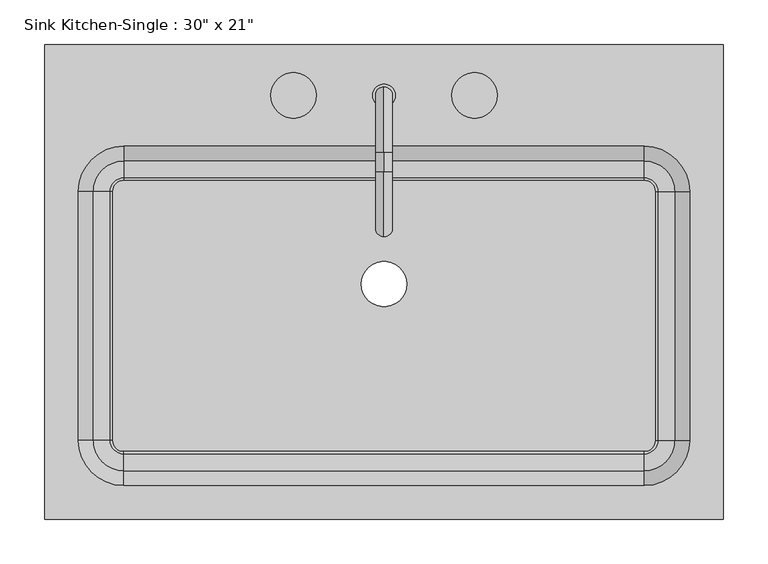
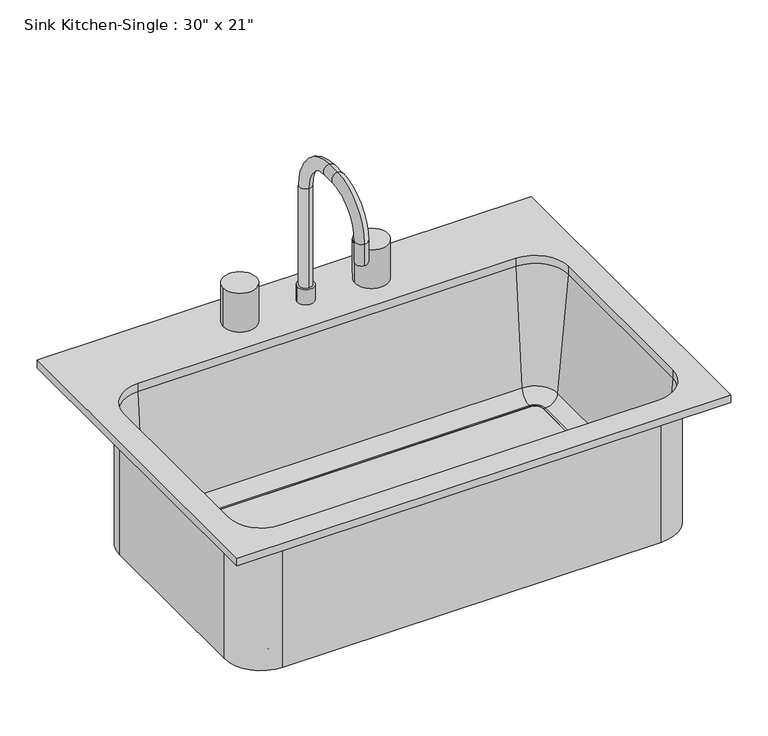
"""IFC4 building model written with IfcOpenShell, lengths in millimetres: flow terminal geometry."""

from ifc_helpers import new_model, si_unit, point, frame, frame_2d, origin, place, context, project, spatial, polyline, circle_curve, ellipse_curve, trimmed, segment, composite_curve, outline, extrude, source, transform, mapped, element, save
from ifc_brep_helpers import plane_surface, cylinder_surface, revolved_surface, advanced_brep


def flow_terminal_38af2918(model_context):
    return source(origin(), model_context, "Body", "SolidModel", [
        advanced_brep(
        [(396.6892406, 269.0454011, 927.1), (-365.3107594, 269.0454011, 927.1), (-365.3107594, -264.3545989, 927.1), (396.6892406, -264.3545989, 927.1), (307.7892406, 154.7454011, 927.1), (358.5892406, 103.9454011, 927.1), (358.5892406, -175.4545989, 927.1), (307.7892406, -226.2545989, 927.1), (-276.4107594, -226.2545989, 927.1), (-327.2107594, -175.4545989, 927.1), (-327.2107594, 103.9454011, 927.1), (-276.4107594, 154.7454011, 927.1), (396.6892406, 269.0454011, 914.4), (396.6892406, -264.3545989, 914.4), (-365.3107594, -264.3545989, 914.4), (-365.3107594, 269.0454011, 914.4), (364.9392406, 103.9454011, 914.4), (307.7892406, 161.0954011, 914.4), (-276.4107594, 161.0954011, 914.4), (-333.5607594, 103.9454011, 914.4), (-333.5607594, -175.4545989, 914.4), (-276.4107594, -232.6045989, 914.4), (307.7892406, -232.6045989, 914.4), (364.9392406, -175.4545989, 914.4), (307.7892406, 154.7454011, 914.4), (358.5892406, 103.9454011, 914.4), (358.5892406, -175.4545989, 914.4), (307.7892406, -226.2545989, 914.4), (-276.4107594, -226.2545989, 914.4), (-327.2107594, -175.4545989, 914.4), (-327.2107594, 103.9454011, 914.4), (-276.4107594, 154.7454011, 914.4), (364.9392406, 103.9454011, 698.5), (307.7892406, 161.0954011, 698.5), (320.4892406, 103.9454011, 698.5), (307.7892406, 116.6454011, 698.5), (320.4892406, 103.9454011, 708.025), (307.7892406, 116.6454011, 708.025), (323.0776588, 103.9454011, 708.025), (307.7892406, 119.2338193, 708.025), (342.0551678, 103.9454011, 725.4146831), (307.7892406, 138.2113283, 725.4146831), (364.9392406, -175.4545989, 698.5), (320.4892406, -175.4545989, 698.5), (320.4892406, -175.4545989, 708.025), (323.0776588, -175.4545989, 708.025), (342.0551678, -175.4545989, 725.4146831), (307.7892406, -232.6045989, 698.5), (307.7892406, -188.1545989, 698.5), (307.7892406, -188.1545989, 708.025), (307.7892406, -190.7430171, 708.025), (307.7892406, -209.7205261, 725.4146831), (-276.4107594, -232.6045989, 698.5), (-276.4107594, -188.1545989, 698.5), (-276.4107594, -188.1545989, 708.025), (-276.4107594, -190.7430171, 708.025), (-276.4107594, -209.7205261, 725.4146831), (-333.5607594, -175.4545989, 698.5), (-289.1107594, -175.4545989, 698.5), (-289.1107594, -175.4545989, 708.025), (-291.6991776, -175.4545989, 708.025), (-310.6766866, -175.4545989, 725.4146831), (-333.5607594, 103.9454011, 698.5), (-289.1107594, 103.9454011, 698.5), (-289.1107594, 103.9454011, 708.025), (-291.6991776, 103.9454011, 708.025), (-310.6766866, 103.9454011, 725.4146831), (-276.4107594, 161.0954011, 698.5), (-276.4107594, 116.6454011, 698.5), (-276.4107594, 116.6454011, 708.025), (-276.4107594, 119.2338193, 708.025), (-276.4107594, 138.2113283, 725.4146831)],
        [
            (0, 1),
            (1, 2),
            (2, 3),
            (3, 0),
            (4, 5, circle_curve(frame((307.7892406, 103.9454011, 927.1), z_axis=(0.0, 0.0, -1.0), x_axis=(1.0, 0.0, 0.0)), 50.8)),
            (5, 6),
            (6, 7, circle_curve(frame((307.7892406, -175.4545989, 927.1), z_axis=(0.0, 0.0, -1.0), x_axis=(1.0, 0.0, 0.0)), 50.8)),
            (7, 8),
            (8, 9, circle_curve(frame((-276.4107594, -175.4545989, 927.1), z_axis=(0.0, 0.0, -1.0), x_axis=(1.0, 0.0, 0.0)), 50.8)),
            (9, 10),
            (10, 11, circle_curve(frame((-276.4107594, 103.9454011, 927.1), z_axis=(0.0, 0.0, -1.0), x_axis=(1.0, 0.0, 0.0)), 50.8)),
            (11, 4),
            (12, 13),
            (13, 14),
            (14, 15),
            (15, 12),
            (16, 17, circle_curve(frame((307.7892406, 103.9454011, 914.4), z_axis=(0.0, 0.0, 1.0), x_axis=(0.0, 1.0, 0.0)), 57.15)),
            (17, 18),
            (18, 19, circle_curve(frame((-276.4107594, 103.9454011, 914.4), z_axis=(0.0, 0.0, 1.0), x_axis=(-1.0, 0.0, 0.0)), 57.15)),
            (19, 20),
            (20, 21, circle_curve(frame((-276.4107594, -175.4545989, 914.4), z_axis=(0.0, 0.0, 1.0), x_axis=(0.0, -1.0, 0.0)), 57.15)),
            (21, 22),
            (22, 23, circle_curve(frame((307.7892406, -175.4545989, 914.4), z_axis=(0.0, 0.0, 1.0), x_axis=(1.0, 0.0, 0.0)), 57.15)),
            (23, 16),
            (0, 12),
            (15, 1),
            (14, 2),
            (13, 3),
            (4, 24),
            (24, 25, circle_curve(frame((307.7892406, 103.9454011, 914.4), z_axis=(0.0, 0.0, -1.0), x_axis=(1.0, 0.0, 0.0)), 50.8)),
            (25, 5),
            (25, 26),
            (26, 6),
            (26, 27, circle_curve(frame((307.7892406, -175.4545989, 914.4), z_axis=(0.0, 0.0, -1.0), x_axis=(1.0, 0.0, 0.0)), 50.8)),
            (27, 7),
            (27, 28),
            (28, 8),
            (28, 29, circle_curve(frame((-276.4107594, -175.4545989, 914.4), z_axis=(0.0, 0.0, -1.0), x_axis=(1.0, 0.0, 0.0)), 50.8)),
            (29, 9),
            (29, 30),
            (30, 10),
            (30, 31, circle_curve(frame((-276.4107594, 103.9454011, 914.4), z_axis=(0.0, 0.0, -1.0), x_axis=(1.0, 0.0, 0.0)), 50.8)),
            (31, 11),
            (31, 24),
            (32, 33, circle_curve(frame((307.7892406, 103.9454011, 698.5), z_axis=(0.0, 0.0, 1.0), x_axis=(0.0, 1.0, 0.0)), 57.15)),
            (33, 17),
            (16, 32),
            (32, 34),
            (34, 35, circle_curve(frame((307.7892406, 103.9454011, 698.5), z_axis=(0.0, 0.0, 1.0), x_axis=(0.0, 1.0, 0.0)), 12.7)),
            (35, 33),
            (34, 36),
            (36, 37, circle_curve(frame((307.7892406, 103.9454011, 708.025), z_axis=(0.0, 0.0, 1.0), x_axis=(0.0, 1.0, 0.0)), 12.7)),
            (37, 35),
            (36, 38),
            (38, 39, circle_curve(frame((307.7892406, 103.9454011, 708.025), z_axis=(0.0, 0.0, 1.0), x_axis=(0.0, 1.0, 0.0)), 15.2884182)),
            (39, 37),
            (38, 40, circle_curve(frame((323.0776588, 103.9454011, 727.075), z_axis=(0.0, -1.0, 0.0), x_axis=(1.0, 0.0, 0.0)), 19.05)),
            (40, 41, circle_curve(frame((307.7892406, 103.9454011, 725.4146831), z_axis=(0.0, 0.0, 1.0), x_axis=(0.0, 1.0, 0.0)), 34.2659272)),
            (41, 39, circle_curve(frame((307.7892406, 119.2338193, 727.075), z_axis=(-1.0, 0.0, 0.0), x_axis=(0.0, 1.0, 0.0)), 19.05)),
            (40, 25),
            (24, 41),
            (23, 42),
            (42, 32),
            (42, 43),
            (43, 34),
            (43, 44),
            (44, 36),
            (44, 45),
            (45, 38),
            (45, 46, circle_curve(frame((323.0776588, -175.4545989, 727.075), z_axis=(0.0, -1.0, 0.0), x_axis=(1.0, 0.0, 0.0)), 19.05)),
            (46, 40),
            (46, 26),
            (22, 47),
            (47, 42, circle_curve(frame((307.7892406, -175.4545989, 698.5), z_axis=(0.0, 0.0, 1.0), x_axis=(1.0, 0.0, 0.0)), 57.15)),
            (47, 48),
            (48, 43, circle_curve(frame((307.7892406, -175.4545989, 698.5), z_axis=(0.0, 0.0, 1.0), x_axis=(1.0, 0.0, 0.0)), 12.7)),
            (48, 49),
            (49, 44, circle_curve(frame((307.7892406, -175.4545989, 708.025), z_axis=(0.0, 0.0, 1.0), x_axis=(1.0, 0.0, 0.0)), 12.7)),
            (49, 50),
            (50, 45, circle_curve(frame((307.7892406, -175.4545989, 708.025), z_axis=(0.0, 0.0, 1.0), x_axis=(1.0, 0.0, 0.0)), 15.2884182)),
            (50, 51, circle_curve(frame((307.7892406, -190.7430171, 727.075), z_axis=(-1.0, 0.0, 0.0), x_axis=(0.0, -1.0, 0.0)), 19.05)),
            (51, 46, circle_curve(frame((307.7892406, -175.4545989, 725.4146831), z_axis=(0.0, 0.0, 1.0), x_axis=(1.0, 0.0, 0.0)), 34.2659272)),
            (51, 27),
            (21, 52),
            (52, 47),
            (52, 53),
            (53, 48),
            (53, 54),
            (54, 49),
            (54, 55),
            (55, 50),
            (55, 56, circle_curve(frame((-276.4107594, -190.7430171, 727.075), z_axis=(-1.0, 0.0, 0.0), x_axis=(0.0, -1.0, 0.0)), 19.05)),
            (56, 51),
            (56, 28),
            (20, 57),
            (57, 52, circle_curve(frame((-276.4107594, -175.4545989, 698.5), z_axis=(0.0, 0.0, 1.0), x_axis=(0.0, -1.0, 0.0)), 57.15)),
            (57, 58),
            (58, 53, circle_curve(frame((-276.4107594, -175.4545989, 698.5), z_axis=(0.0, 0.0, 1.0), x_axis=(0.0, -1.0, 0.0)), 12.7)),
            (58, 59),
            (59, 54, circle_curve(frame((-276.4107594, -175.4545989, 708.025), z_axis=(0.0, 0.0, 1.0), x_axis=(0.0, -1.0, 0.0)), 12.7)),
            (59, 60),
            (60, 55, circle_curve(frame((-276.4107594, -175.4545989, 708.025), z_axis=(0.0, 0.0, 1.0), x_axis=(0.0, -1.0, 0.0)), 15.2884182)),
            (60, 61, circle_curve(frame((-291.6991776, -175.4545989, 727.075), z_axis=(0.0, 1.0, 0.0), x_axis=(-1.0, 0.0, 0.0)), 19.05)),
            (61, 56, circle_curve(frame((-276.4107594, -175.4545989, 725.4146831), z_axis=(0.0, 0.0, 1.0), x_axis=(0.0, -1.0, 0.0)), 34.2659272)),
            (61, 29),
            (19, 62),
            (62, 57),
            (62, 63),
            (63, 58),
            (63, 64),
            (64, 59),
            (64, 65),
            (65, 60),
            (65, 66, circle_curve(frame((-291.6991776, 103.9454011, 727.075), z_axis=(0.0, 1.0, 0.0), x_axis=(-1.0, 0.0, 0.0)), 19.05)),
            (66, 61),
            (66, 30),
            (18, 67),
            (67, 62, circle_curve(frame((-276.4107594, 103.9454011, 698.5), z_axis=(0.0, 0.0, 1.0), x_axis=(-1.0, 0.0, 0.0)), 57.15)),
            (67, 68),
            (68, 63, circle_curve(frame((-276.4107594, 103.9454011, 698.5), z_axis=(0.0, 0.0, 1.0), x_axis=(-1.0, 0.0, 0.0)), 12.7)),
            (68, 69),
            (69, 64, circle_curve(frame((-276.4107594, 103.9454011, 708.025), z_axis=(0.0, 0.0, 1.0), x_axis=(-1.0, 0.0, 0.0)), 12.7)),
            (69, 70),
            (70, 65, circle_curve(frame((-276.4107594, 103.9454011, 708.025), z_axis=(0.0, 0.0, 1.0), x_axis=(-1.0, 0.0, 0.0)), 15.2884182)),
            (70, 71, circle_curve(frame((-276.4107594, 119.2338193, 727.075), z_axis=(1.0, 0.0, 0.0), x_axis=(0.0, 1.0, 0.0)), 19.05)),
            (71, 66, circle_curve(frame((-276.4107594, 103.9454011, 725.4146831), z_axis=(0.0, 0.0, 1.0), x_axis=(-1.0, 0.0, 0.0)), 34.2659272)),
            (71, 31),
            (33, 67),
            (35, 68),
            (37, 69),
            (39, 70),
            (41, 71),
        ],
        [
            plane_surface(frame((-365.3107594, 269.0454011, 927.1), z_axis=(0.0, 0.0, 1.0), x_axis=(-1.0, 0.0, 0.0))),
            plane_surface(frame((-365.3107594, 269.0454011, 914.4), z_axis=(0.0, 0.0, -1.0), x_axis=(1.0, 0.0, 0.0))),
            plane_surface(frame((396.6892406, 269.0454011, 927.1), z_axis=(0.0, 1.0, 0.0), x_axis=(0.0, 0.0, -1.0))),
            plane_surface(frame((-365.3107594, 269.0454011, 927.1), z_axis=(-1.0, 0.0, 0.0), x_axis=(0.0, 0.0, -1.0))),
            plane_surface(frame((-365.3107594, -264.3545989, 927.1), z_axis=(0.0, -1.0, 0.0), x_axis=(0.0, 0.0, -1.0))),
            plane_surface(frame((396.6892406, -264.3545989, 927.1), z_axis=(1.0, 0.0, 0.0), x_axis=(0.0, 0.0, -1.0))),
            revolved_surface(polyline([(358.58924060000004, 103.9454011, 914.4), (358.58924060000004, 103.9454011, 927.1)]), (307.7892406, 103.9454011, 0.0), (0.0, 0.0, -1.0)),
            plane_surface(frame((358.5892406, 103.9454011, 927.1), z_axis=(-1.0, 0.0, 0.0), x_axis=(0.0, 0.0, -1.0))),
            revolved_surface(polyline([(358.58924060000004, -175.4545989, 914.4), (358.58924060000004, -175.4545989, 927.1)]), (307.7892406, -175.4545989, 0.0), (0.0, 0.0, -1.0)),
            plane_surface(frame((307.7892406, -226.2545989, 927.1), z_axis=(0.0, 1.0, 0.0), x_axis=(0.0, 0.0, -1.0))),
            revolved_surface(polyline([(-225.6107594, -175.4545989, 914.4), (-225.6107594, -175.4545989, 927.1)]), (-276.4107594, -175.4545989, 0.0), (0.0, 0.0, -1.0)),
            plane_surface(frame((-327.2107594, -175.4545989, 927.1), z_axis=(1.0, 0.0, 0.0), x_axis=(0.0, 0.0, -1.0))),
            revolved_surface(polyline([(-225.6107594, 103.9454011, 914.4), (-225.6107594, 103.9454011, 927.1)]), (-276.4107594, 103.9454011, 0.0), (0.0, 0.0, -1.0)),
            plane_surface(frame((-276.4107594, 154.7454011, 927.1), z_axis=(0.0, -1.0, 0.0), x_axis=(0.0, 0.0, -1.0))),
            cylinder_surface(frame((307.7892406, 103.9454011, 0.0), z_axis=(0.0, 0.0, -1.0), x_axis=(0.0, 1.0, 0.0)), 57.15),
            plane_surface(frame((307.7892406, 103.9454011, 698.5), z_axis=(0.0, 0.0, -1.0), x_axis=(0.0, 1.0, 0.0))),
            revolved_surface(polyline([(307.7892406, 116.6454011, 698.5), (307.7892406, 116.6454011, 708.025)]), (307.7892406, 103.9454011, 0.0), (0.0, 0.0, -1.0)),
            plane_surface(frame((307.7892406, 103.9454011, 708.025), z_axis=(0.0, 0.0, 1.0), x_axis=(0.0, 1.0, 0.0))),
            revolved_surface(trimmed(ellipse_curve(frame((307.7892406, 119.2338193, 727.075), z_axis=(1.0, 0.0, 0.0), x_axis=(0.0, 1.0, 0.0)), 19.05, 19.05), [point((307.7892406, 119.2338193, 708.025))], [point((307.7892406, 138.2113283, 725.4146831))], True, "CARTESIAN"), (307.7892406, 103.9454011, 0.0), (0.0, 0.0, -1.0)),
            revolved_surface(polyline([(307.7892406, 138.2113283, 725.4146831), (307.7892406, 154.7454011, 914.4)]), (307.7892406, 103.9454011, 0.0), (0.0, 0.0, -1.0)),
            plane_surface(frame((364.9392406, 103.9454011, 914.4), z_axis=(1.0, 0.0, 0.0), x_axis=(0.0, -1.0, 0.0))),
            plane_surface(frame((364.9392406, 103.9454011, 698.5), z_axis=(0.0, 0.0, -1.0), x_axis=(0.0, -1.0, 0.0))),
            plane_surface(frame((320.4892406, 103.9454011, 698.5), z_axis=(-1.0, 0.0, 0.0), x_axis=(0.0, -1.0, 0.0))),
            plane_surface(frame((320.4892406, 103.9454011, 708.025), z_axis=(0.0, 0.0, 1.0), x_axis=(0.0, -1.0, 0.0))),
            revolved_surface(polyline([(342.1276588, -175.45459889999998, 727.075), (342.1276588, 103.9454011, 727.075)]), (323.0776588, 103.9454011, 727.075), (0.0, -1.0, 0.0)),
            plane_surface(frame((342.0551678, 103.9454011, 725.4146831), z_axis=(-0.9961946980917442, 0.0, 0.08715574274767306), x_axis=(0.0, -1.0, 0.0))),
            cylinder_surface(frame((307.7892406, -175.4545989, 0.0), z_axis=(0.0, 0.0, -1.0), x_axis=(1.0, 0.0, 0.0)), 57.15),
            plane_surface(frame((307.7892406, -175.4545989, 698.5), z_axis=(0.0, 0.0, -1.0), x_axis=(1.0, 0.0, 0.0))),
            revolved_surface(polyline([(320.4892406, -175.4545989, 698.5), (320.4892406, -175.4545989, 708.025)]), (307.7892406, -175.4545989, 0.0), (0.0, 0.0, -1.0)),
            plane_surface(frame((307.7892406, -175.4545989, 708.025), z_axis=(0.0, 0.0, 1.0), x_axis=(1.0, 0.0, 0.0))),
            revolved_surface(trimmed(ellipse_curve(frame((323.0776588, -175.4545989, 727.075), z_axis=(0.0, -1.0, 0.0), x_axis=(1.0, 0.0, 0.0)), 19.05, 19.05), [point((323.0776588, -175.4545989, 708.025))], [point((342.0551678, -175.4545989, 725.4146831))], True, "CARTESIAN"), (307.7892406, -175.4545989, 0.0), (0.0, 0.0, -1.0)),
            revolved_surface(polyline([(342.0551678, -175.4545989, 725.4146831), (358.5892406, -175.4545989, 914.4)]), (307.7892406, -175.4545989, 0.0), (0.0, 0.0, -1.0)),
            plane_surface(frame((307.7892406, -232.6045989, 914.4), z_axis=(0.0, -1.0, 0.0), x_axis=(-1.0, 0.0, 0.0))),
            plane_surface(frame((307.7892406, -232.6045989, 698.5), z_axis=(0.0, 0.0, -1.0), x_axis=(-1.0, 0.0, 0.0))),
            plane_surface(frame((307.7892406, -188.1545989, 698.5), z_axis=(0.0, 1.0, 0.0), x_axis=(-1.0, 0.0, 0.0))),
            plane_surface(frame((307.7892406, -188.1545989, 708.025), z_axis=(0.0, 0.0, 1.0), x_axis=(-1.0, 0.0, 0.0))),
            revolved_surface(polyline([(-276.4107594, -209.79301710000001, 727.075), (307.7892406, -209.79301710000001, 727.075)]), (307.7892406, -190.7430171, 727.075), (-1.0, 0.0, 0.0)),
            plane_surface(frame((307.7892406, -209.7205261, 725.4146831), z_axis=(0.0, 0.9961946980917442, 0.08715574274767306), x_axis=(-1.0, 0.0, 0.0))),
            cylinder_surface(frame((-276.4107594, -175.4545989, 0.0), z_axis=(0.0, 0.0, -1.0), x_axis=(0.0, -1.0, 0.0)), 57.15),
            plane_surface(frame((-276.4107594, -175.4545989, 698.5), z_axis=(0.0, 0.0, -1.0), x_axis=(0.0, -1.0, 0.0))),
            revolved_surface(polyline([(-276.4107594, -188.1545989, 698.5), (-276.4107594, -188.1545989, 708.025)]), (-276.4107594, -175.4545989, 0.0), (0.0, 0.0, -1.0)),
            plane_surface(frame((-276.4107594, -175.4545989, 708.025), z_axis=(0.0, 0.0, 1.0), x_axis=(0.0, -1.0, 0.0))),
            revolved_surface(trimmed(ellipse_curve(frame((-276.4107594, -190.7430171, 727.075), z_axis=(-1.0, 0.0, 0.0), x_axis=(0.0, -1.0, 0.0)), 19.05, 19.05), [point((-276.4107594, -190.7430171, 708.025))], [point((-276.4107594, -209.7205261, 725.4146831))], True, "CARTESIAN"), (-276.4107594, -175.4545989, 0.0), (0.0, 0.0, -1.0)),
            revolved_surface(polyline([(-276.4107594, -209.7205261, 725.4146831), (-276.4107594, -226.2545989, 914.4)]), (-276.4107594, -175.4545989, 0.0), (0.0, 0.0, -1.0)),
            plane_surface(frame((-333.5607594, -175.4545989, 914.4), z_axis=(-1.0, 0.0, 0.0), x_axis=(0.0, 1.0, 0.0))),
            plane_surface(frame((-333.5607594, -175.4545989, 698.5), z_axis=(0.0, 0.0, -1.0), x_axis=(0.0, 1.0, 0.0))),
            plane_surface(frame((-289.1107594, -175.4545989, 698.5), z_axis=(1.0, 0.0, 0.0), x_axis=(0.0, 1.0, 0.0))),
            plane_surface(frame((-289.1107594, -175.4545989, 708.025), z_axis=(0.0, 0.0, 1.0), x_axis=(0.0, 1.0, 0.0))),
            revolved_surface(polyline([(-310.7491776, 103.94540109999997, 727.075), (-310.7491776, -175.4545989, 727.075)]), (-291.6991776, -175.4545989, 727.075), (0.0, 1.0, 0.0)),
            plane_surface(frame((-310.6766866, -175.4545989, 725.4146831), z_axis=(0.9961946980917442, 0.0, 0.08715574274767306), x_axis=(0.0, 1.0, 0.0))),
            cylinder_surface(frame((-276.4107594, 103.9454011, 0.0), z_axis=(0.0, 0.0, -1.0), x_axis=(-1.0, 0.0, 0.0)), 57.15),
            plane_surface(frame((-276.4107594, 103.9454011, 698.5), z_axis=(0.0, 0.0, -1.0), x_axis=(-1.0, 0.0, 0.0))),
            revolved_surface(polyline([(-289.1107594, 103.9454011, 698.5), (-289.1107594, 103.9454011, 708.025)]), (-276.4107594, 103.9454011, 0.0), (0.0, 0.0, -1.0)),
            plane_surface(frame((-276.4107594, 103.9454011, 708.025), z_axis=(0.0, 0.0, 1.0), x_axis=(-1.0, 0.0, 0.0))),
            revolved_surface(trimmed(ellipse_curve(frame((-291.6991776, 103.9454011, 727.075), z_axis=(0.0, 1.0, 0.0), x_axis=(-1.0, 0.0, 0.0)), 19.05, 19.05), [point((-291.6991776, 103.9454011, 708.025))], [point((-310.6766866, 103.9454011, 725.4146831))], True, "CARTESIAN"), (-276.4107594, 103.9454011, 0.0), (0.0, 0.0, -1.0)),
            revolved_surface(polyline([(-310.6766866, 103.9454011, 725.4146831), (-327.2107594, 103.9454011, 914.4)]), (-276.4107594, 103.9454011, 0.0), (0.0, 0.0, -1.0)),
            plane_surface(frame((-276.4107594, 161.0954011, 914.4), z_axis=(0.0, 1.0, 0.0), x_axis=(1.0, 0.0, 0.0))),
            plane_surface(frame((-276.4107594, 161.0954011, 698.5), z_axis=(0.0, 0.0, -1.0), x_axis=(1.0, 0.0, 0.0))),
            plane_surface(frame((-276.4107594, 116.6454011, 698.5), z_axis=(0.0, -1.0, 0.0), x_axis=(1.0, 0.0, 0.0))),
            plane_surface(frame((-276.4107594, 116.6454011, 708.025), z_axis=(0.0, 0.0, 1.0), x_axis=(1.0, 0.0, 0.0))),
            revolved_surface(polyline([(307.7892406, 138.2838193, 727.075), (-276.4107594, 138.2838193, 727.075)]), (-276.4107594, 119.2338193, 727.075), (1.0, 0.0, 0.0)),
            plane_surface(frame((-276.4107594, 138.2113283, 725.4146831), z_axis=(0.0, -0.9961946980917442, 0.08715574274767306), x_axis=(1.0, 0.0, 0.0))),
        ],
        [
            (0, [[1, 2, 3, 4], [5, 6, 7, 8, 9, 10, 11, 12]]),
            (1, [[13, 14, 15, 16], [17, 18, 19, 20, 21, 22, 23, 24]]),
            (2, [[-1, 25, -16, 26]]),
            (3, [[-2, -26, -15, 27]]),
            (4, [[-3, -27, -14, 28]]),
            (5, [[-4, -28, -13, -25]]),
            (6, [[-5, 29, 30, 31]]),
            (7, [[-6, -31, 32, 33]]),
            (8, [[-7, -33, 34, 35]]),
            (9, [[-8, -35, 36, 37]]),
            (10, [[-9, -37, 38, 39]]),
            (11, [[-10, -39, 40, 41]]),
            (12, [[-11, -41, 42, 43]]),
            (13, [[-12, -43, 44, -29]]),
            (14, [[45, 46, -17, 47]]),
            (15, [[-45, 48, 49, 50]]),
            (16, [[-49, 51, 52, 53]]),
            (17, [[-52, 54, 55, 56]]),
            (18, [[-55, 57, 58, 59]]),
            (19, [[-58, 60, -30, 61]]),
            (20, [[-47, -24, 62, 63]]),
            (21, [[-48, -63, 64, 65]]),
            (22, [[-51, -65, 66, 67]]),
            (23, [[-54, -67, 68, 69]]),
            (24, [[-57, -69, 70, 71]]),
            (25, [[-60, -71, 72, -32]]),
            (26, [[-62, -23, 73, 74]]),
            (27, [[-64, -74, 75, 76]]),
            (28, [[-66, -76, 77, 78]]),
            (29, [[-68, -78, 79, 80]]),
            (30, [[-70, -80, 81, 82]]),
            (31, [[-72, -82, 83, -34]]),
            (32, [[-73, -22, 84, 85]]),
            (33, [[-75, -85, 86, 87]]),
            (34, [[-77, -87, 88, 89]]),
            (35, [[-79, -89, 90, 91]]),
            (36, [[-81, -91, 92, 93]]),
            (37, [[-83, -93, 94, -36]]),
            (38, [[-84, -21, 95, 96]]),
            (39, [[-86, -96, 97, 98]]),
            (40, [[-88, -98, 99, 100]]),
            (41, [[-90, -100, 101, 102]]),
            (42, [[-92, -102, 103, 104]]),
            (43, [[-94, -104, 105, -38]]),
            (44, [[-95, -20, 106, 107]]),
            (45, [[-97, -107, 108, 109]]),
            (46, [[-99, -109, 110, 111]]),
            (47, [[-101, -111, 112, 113]]),
            (48, [[-103, -113, 114, 115]]),
            (49, [[-105, -115, 116, -40]]),
            (50, [[-106, -19, 117, 118]]),
            (51, [[-108, -118, 119, 120]]),
            (52, [[-110, -120, 121, 122]]),
            (53, [[-112, -122, 123, 124]]),
            (54, [[-114, -124, 125, 126]]),
            (55, [[-116, -126, 127, -42]]),
            (56, [[-46, 128, -117, -18]]),
            (57, [[-50, 129, -119, -128]]),
            (58, [[-53, 130, -121, -129]]),
            (59, [[-56, 131, -123, -130]]),
            (60, [[-59, 132, -125, -131]]),
            (61, [[-61, -44, -127, -132]]),
        ],
    ),
        advanced_brep(
        [(2.9892406, 211.8954011, 927.1), (28.3892406, 211.8954011, 927.1), (15.6892406, 221.4204011, 1114.425), (15.6892406, 202.3704011, 1114.425), (15.6892406, 202.3704011, 952.5), (15.6892406, 221.4204011, 952.5), (15.6892406, 148.3954011, 1187.45), (15.6892406, 148.3954011, 1168.4), (15.6892406, 126.1704011, 1187.45), (15.6892406, 126.1704011, 1168.4), (15.6892406, 53.1454011, 1114.425), (15.6892406, 72.1954011, 1114.425), (15.6892406, 53.1454011, 1079.5), (15.6892406, 72.1954011, 1079.5), (2.9892406, 211.8954011, 952.5), (28.3892406, 211.8954011, 952.5)],
        [
            (0, 1, circle_curve(frame((15.6892406, 211.8954011, 927.1), z_axis=(0.0, 0.0, -1.0), x_axis=(1.0, 0.0, 0.0)), 12.7)),
            (1, 0, circle_curve(frame((15.6892406, 211.8954011, 927.1), z_axis=(0.0, 0.0, -1.0), x_axis=(1.0, 0.0, 0.0)), 12.7)),
            (2, 3, circle_curve(frame((15.6892406, 211.8954011, 1114.425), z_axis=(0.0, 0.0, -1.0), x_axis=(0.0, -1.0, 0.0)), 9.525)),
            (3, 4),
            (4, 5, circle_curve(frame((15.6892406, 211.8954011, 952.5), z_axis=(0.0, 0.0, 1.0), x_axis=(0.0, -1.0, 0.0)), 9.525)),
            (5, 2),
            (3, 2, circle_curve(frame((15.6892406, 211.8954011, 1114.425), z_axis=(0.0, 0.0, -1.0), x_axis=(0.0, -1.0, 0.0)), 9.525)),
            (5, 4, circle_curve(frame((15.6892406, 211.8954011, 952.5), z_axis=(0.0, 0.0, 1.0), x_axis=(0.0, -1.0, 0.0)), 9.525)),
            (2, 6, circle_curve(frame((15.6892406, 148.3954011, 1114.425), z_axis=(1.0, 0.0, 0.0), x_axis=(0.0, 1.0, 0.0)), 73.025)),
            (6, 7, circle_curve(frame((15.6892406, 148.3954011, 1177.925), z_axis=(0.0, 1.0, 0.0), x_axis=(0.0, 0.0, -1.0)), 9.525)),
            (7, 3, circle_curve(frame((15.6892406, 148.3954011, 1114.425), z_axis=(-1.0, 0.0, 0.0), x_axis=(0.0, 1.0, 0.0)), 53.975)),
            (7, 6, circle_curve(frame((15.6892406, 148.3954011, 1177.925), z_axis=(0.0, 1.0, 0.0), x_axis=(0.0, 0.0, -1.0)), 9.525)),
            (6, 8),
            (8, 9, circle_curve(frame((15.6892406, 126.1704011, 1177.925), z_axis=(0.0, 1.0, 0.0), x_axis=(0.0, 0.0, -1.0)), 9.525)),
            (9, 7),
            (9, 8, circle_curve(frame((15.6892406, 126.1704011, 1177.925), z_axis=(0.0, 1.0, 0.0), x_axis=(0.0, 0.0, -1.0)), 9.525)),
            (8, 10, circle_curve(frame((15.6892406, 126.1704011, 1114.425), z_axis=(1.0, 0.0, 0.0), x_axis=(0.0, 0.0, 1.0)), 73.025)),
            (10, 11, circle_curve(frame((15.6892406, 62.6704011, 1114.425), z_axis=(0.0, 0.0, 1.0), x_axis=(0.0, 1.0, 0.0)), 9.525)),
            (11, 9, circle_curve(frame((15.6892406, 126.1704011, 1114.425), z_axis=(-1.0, 0.0, 0.0), x_axis=(0.0, 0.0, 1.0)), 53.975)),
            (11, 10, circle_curve(frame((15.6892406, 62.6704011, 1114.425), z_axis=(0.0, 0.0, 1.0), x_axis=(0.0, 1.0, 0.0)), 9.525)),
            (12, 13, circle_curve(frame((15.6892406, 62.6704011, 1079.5), z_axis=(0.0, 0.0, -1.0), x_axis=(0.0, 1.0, 0.0)), 9.525)),
            (13, 12, circle_curve(frame((15.6892406, 62.6704011, 1079.5), z_axis=(0.0, 0.0, -1.0), x_axis=(0.0, 1.0, 0.0)), 9.525)),
            (10, 12),
            (13, 11),
            (14, 15, circle_curve(frame((15.6892406, 211.8954011, 952.5), z_axis=(0.0, 0.0, 1.0), x_axis=(1.0, 0.0, 0.0)), 12.7)),
            (15, 14, circle_curve(frame((15.6892406, 211.8954011, 952.5), z_axis=(0.0, 0.0, 1.0), x_axis=(1.0, 0.0, 0.0)), 12.7)),
            (14, 0),
            (1, 15),
        ],
        [
            plane_surface(frame((15.6892406, 202.3704011, 927.1), z_axis=(0.0, 0.0, -1.0), x_axis=(1.0, 0.0, 0.0))),
            cylinder_surface(frame((15.6892406, 211.8954011, 927.1), z_axis=(0.0, 0.0, -1.0), x_axis=(0.0, -1.0, 0.0)), 9.525),
            revolved_surface(trimmed(ellipse_curve(frame((15.6892406, 211.8954011, 1114.425), z_axis=(0.0, 0.0, -1.0), x_axis=(0.0, -1.0, 0.0)), 9.525, 9.525), [point((15.6892406, 221.4204011, 1114.425))], [point((15.6892406, 202.3704011, 1114.425))], True, "CARTESIAN"), (15.6892406, 148.3954011, 1114.425), (1.0, 0.0, 0.0)),
            revolved_surface(trimmed(ellipse_curve(frame((15.6892406, 211.8954011, 1114.425), z_axis=(0.0, 0.0, -1.0), x_axis=(0.0, -1.0, 0.0)), 9.525, 9.525), [point((15.6892406, 202.3704011, 1114.425))], [point((15.6892406, 221.4204011, 1114.425))], True, "CARTESIAN"), (15.6892406, 148.3954011, 1114.425), (1.0, 0.0, 0.0)),
            cylinder_surface(frame((15.6892406, 148.3954011, 1177.925), z_axis=(0.0, 1.0, 0.0), x_axis=(0.0, 0.0, -1.0)), 9.525),
            revolved_surface(trimmed(ellipse_curve(frame((15.6892406, 126.1704011, 1177.925), z_axis=(0.0, 1.0, 0.0), x_axis=(0.0, 0.0, -1.0)), 9.525, 9.525), [point((15.6892406, 126.1704011, 1187.45))], [point((15.6892406, 126.1704011, 1168.4))], True, "CARTESIAN"), (15.6892406, 126.1704011, 1114.425), (1.0, 0.0, 0.0)),
            revolved_surface(trimmed(ellipse_curve(frame((15.6892406, 126.1704011, 1177.925), z_axis=(0.0, 1.0, 0.0), x_axis=(0.0, 0.0, -1.0)), 9.525, 9.525), [point((15.6892406, 126.1704011, 1168.4))], [point((15.6892406, 126.1704011, 1187.45))], True, "CARTESIAN"), (15.6892406, 126.1704011, 1114.425), (1.0, 0.0, 0.0)),
            plane_surface(frame((15.6892406, 53.1454011, 1079.5), z_axis=(0.0, 0.0, -1.0), x_axis=(-1.0, 0.0, 0.0))),
            cylinder_surface(frame((15.6892406, 62.6704011, 1114.425), z_axis=(0.0, 0.0, 1.0), x_axis=(0.0, 1.0, 0.0)), 9.525),
            plane_surface(frame((28.3892406, 211.8954011, 952.5), z_axis=(0.0, 0.0, 1.0), x_axis=(0.0, 1.0, 0.0))),
            cylinder_surface(frame((15.6892406, 211.8954011, 927.1), z_axis=(0.0, 0.0, 1.0), x_axis=(1.0, 0.0, 0.0)), 12.7),
        ],
        [
            (0, [[1, 2]]),
            (1, [[3, 4, 5, 6]]),
            (1, [[7, -6, 8, -4]]),
            (2, [[-3, 9, 10, 11]]),
            (3, [[-7, -11, 12, -9]]),
            (4, [[-10, 13, 14, 15]]),
            (4, [[-12, -15, 16, -13]]),
            (5, [[-14, 17, 18, 19]]),
            (6, [[-16, -19, 20, -17]]),
            (7, [[21, 22]]),
            (8, [[-18, 23, -22, 24]]),
            (8, [[-20, -24, -21, -23]]),
            (9, [[25, 26], [-5, -8]]),
            (10, [[-25, 27, -2, 28]]),
            (10, [[-26, -28, -1, -27]]),
        ],
    ),
        extrude(outline(composite_curve([segment(trimmed(circle_curve(frame_2d((-85.9107594, 211.8954011)), 25.4), [point((-111.3107594, 211.8954011))], [point((-60.5107594, 211.8954011))], False, "CARTESIAN"), True, "CONTINUOUS"), segment(trimmed(circle_curve(frame_2d((-85.9107594, 211.8954011)), 25.4), [point((-60.5107594, 211.8954011))], [point((-111.3107594, 211.8954011))], False, "CARTESIAN"), True, "CONTINUOUS")], self_intersect=False)), frame((0.0, 0.0, 927.1), z_axis=(0.0, 0.0, 1.0), x_axis=(1.0, 0.0, 0.0)), (0.0, 0.0, 1.0), 63.5),
        extrude(outline(composite_curve([segment(trimmed(circle_curve(frame_2d((117.2892406, 211.8954011)), 25.4), [point((91.8892406, 211.8954011))], [point((142.6892406, 211.8954011))], False, "CARTESIAN"), True, "CONTINUOUS"), segment(trimmed(circle_curve(frame_2d((117.2892406, 211.8954011)), 25.4), [point((142.6892406, 211.8954011))], [point((91.8892406, 211.8954011))], False, "CARTESIAN"), True, "CONTINUOUS")], self_intersect=False)), frame((0.0, 0.0, 927.1), z_axis=(0.0, 0.0, 1.0), x_axis=(1.0, 0.0, 0.0)), (0.0, 0.0, 1.0), 63.5),
        extrude(outline(composite_curve([segment(trimmed(circle_curve(frame_2d((307.7892406, 103.9454011)), 12.7), [point((307.7892406, 116.6454011))], [point((320.4892406, 103.9454011))], False, "CARTESIAN"), True, "CONTINUOUS"), segment(polyline([(320.4892406, 103.9454011), (320.4892406, -175.4545989)]), True, "CONTINUOUS"), segment(trimmed(circle_curve(frame_2d((307.7892406, -175.4545989)), 12.7), [point((320.4892406, -175.4545989))], [point((307.7892406, -188.1545989))], False, "CARTESIAN"), True, "CONTINUOUS"), segment(polyline([(307.7892406, -188.1545989), (-276.4107594, -188.1545989)]), True, "CONTINUOUS"), segment(trimmed(circle_curve(frame_2d((-276.4107594, -175.4545989)), 12.7), [point((-276.4107594, -188.1545989))], [point((-289.1107594, -175.4545989))], False, "CARTESIAN"), True, "CONTINUOUS"), segment(polyline([(-289.1107594, -175.4545989), (-289.1107594, 103.9454011)]), True, "CONTINUOUS"), segment(trimmed(circle_curve(frame_2d((-276.4107594, 103.9454011)), 12.7), [point((-289.1107594, 103.9454011))], [point((-276.4107594, 116.6454011))], False, "CARTESIAN"), True, "CONTINUOUS"), segment(polyline([(-276.4107594, 116.6454011), (307.7892406, 116.6454011)]), True, "CONTINUOUS")], self_intersect=False), holes=[composite_curve([segment(trimmed(circle_curve(frame_2d((15.6892406, 0.0)), 25.4), [point((-9.7107594, 0.0))], [point((41.0892406, 0.0))], True, "CARTESIAN"), True, "CONTINUOUS"), segment(trimmed(circle_curve(frame_2d((15.6892406, 0.0)), 25.4), [point((41.0892406, 0.0))], [point((-9.7107594, 0.0))], True, "CARTESIAN"), True, "CONTINUOUS")], self_intersect=False)]), frame((0.0, 0.0, 698.5), z_axis=(0.0, 0.0, 1.0), x_axis=(1.0, 0.0, 0.0)), (0.0, 0.0, 1.0), 9.525),
    ])


if __name__ == "__main__":
    model = new_model("IFC4")
    model_context = context("Model", 3, world=origin())
    ifc_project = project(units=[si_unit("LENGTHUNIT", "METRE", prefix="MILLI")], contexts=[model_context])
    site = spatial("IfcSite", under=ifc_project)
    building = spatial("IfcBuilding", under=site)
    placement = place(None, origin())
    flow_terminal_shape = flow_terminal_38af2918(model_context)
    element("IfcFlowTerminal", 1, ObjectType="Sink Kitchen-Single : 30\" x 21\"", at=placement, inside=building, context=model_context, shape_type="MappedRepresentation", body=[
        mapped(flow_terminal_shape, transform((0.0, 0.0, 0.0), x_axis=(1.0, 0.0, 0.0), y_axis=(0.0, 1.0, 0.0), z_axis=(0.0, 0.0, 1.0))),
    ])
    save(model, "model.ifc")

# Revit data of these elements
# Type "Sink Kitchen-Single : 30\" x 21\""
#   Assembly Code = "D2010410"
#   Counter Height = 3' - 0"
#   Depth = 1' - 9"
#   Width = 2' - 6"
#   Faucet Material = Steel, Polished
#   Sink Material = Steel, Polished
#   Default Elevation = 0
# Element 1 (IfcFlowTerminal, "Sink Kitchen-Single : 30\" x 21\"")
#   Materials on its faces: "Steel, Polished"
# Materials
#   "Steel, Polished": class "Metal", colour RGB 57 57 57, transparency 0, Description = "Polished steel", Cost = 0
